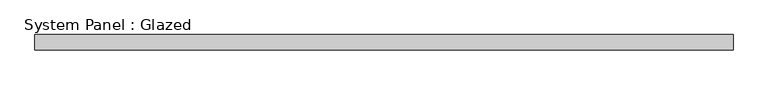
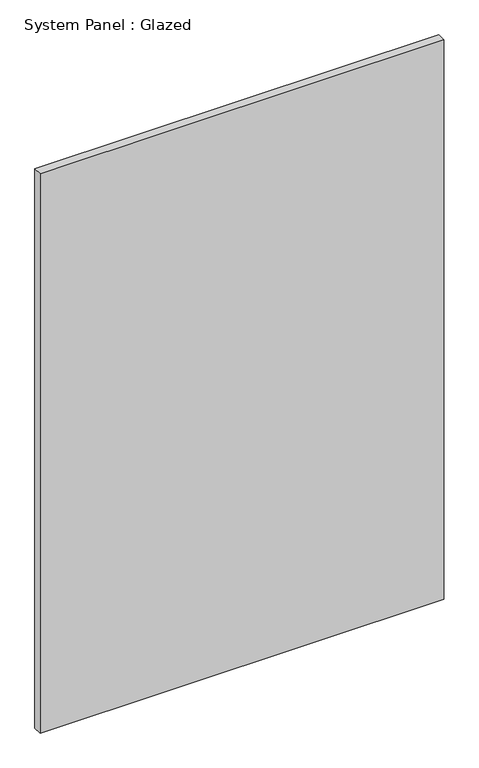
"""IFC4 building model written with IfcOpenShell, lengths in millimetres: plate geometry, System Panel : Glazed."""

from ifc_helpers import new_model, si_unit, origin, origin_with_axes, place, context, project, spatial, polyline, outline, extrude, source, transform, mapped, element, save


def system_panel_glazed_1e1b7e15(model_context):
    return source(origin(), model_context, "Body", "SweptSolid", [
        extrude(outline(polyline([(581.025, -44.45), (-581.025, -44.45), (-581.025, -19.05), (581.025, -19.05), (581.025, -44.45)])), origin_with_axes(), (0.0, 0.0, 1.0), 1701.8),
    ])


if __name__ == "__main__":
    model = new_model("IFC4")
    model_context = context("Model", 3, world=origin())
    ifc_project = project(units=[si_unit("LENGTHUNIT", "METRE", prefix="MILLI")], contexts=[model_context])
    site = spatial("IfcSite", under=ifc_project)
    building = spatial("IfcBuilding", under=site)
    placement = place(None, origin())
    system_panel_glazed_shape = system_panel_glazed_1e1b7e15(model_context)
    element("IfcPlate", 1, ObjectType="System Panel : Glazed", at=placement, inside=building, context=model_context, shape_type="MappedRepresentation", body=[
        mapped(system_panel_glazed_shape, transform((0.0, 0.0, 0.0), x_axis=(1.0, 0.0, 0.0), y_axis=(0.0, 1.0, 0.0), z_axis=(0.0, 0.0, 1.0))),
    ])
    save(model, "model.ifc")

# Revit data of these elements
# Type "System Panel : Glazed"
#   Construction Type Id = "GSP4R"
#   Analytic Construction = "1/8 in Pilkington single glazing"
#   Visual Light Transmittance = 0.9
#   Solar Heat Gain Coefficient = 0.86
#   Heat Transfer Coefficient (U) = 1.18115 BTU/(h·ft²·°F)
#   Define Thermal Properties by = 1
# Element 1 (IfcPlate, "System Panel : Glazed")
#   Materials on its faces: "Glass"
# Materials
#   "Glass": class "Glass", colour RGB 0 128 192, transparency 0.75, Description = "Soda Lime Glass", Cost = 0
